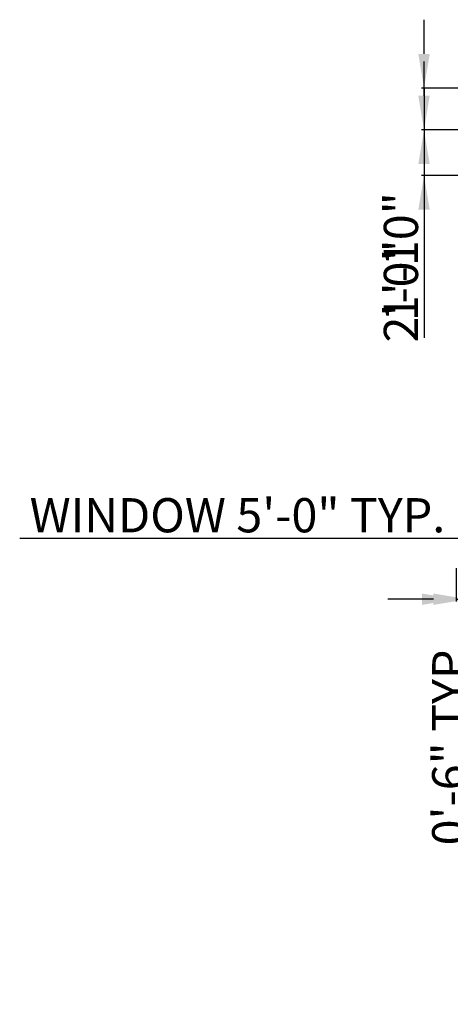
# Model space of a CAD drawing. Units: inches. Extents: x -261 to 409, y 193 to 762.
# Tile 1 of 6: x -261 to -35, y 193 to 711. Entities that reach past the tile are written whole.
import ezdxf

# ---------------------------------------------------------------- set-up
doc = ezdxf.new("R2010")
doc.units = ezdxf.units.IN
doc.layers.add('A-ANNO-DIMS', color=2, linetype='Continuous', lineweight=18)
doc.styles.get("Standard").update_dxf_attribs({"font": 'arial.ttf'})
doc.dimstyles.new('ISO-25', dxfattribs={"dimtxt": 18, "dimasz": 18, "dimexe": 1.25, "dimexo": 0.625, "dimtad": 1, "dimdec": 1, "dimlunit": 3, "dimtxsty": 'Standard', "dimcen": 2.5, "dimadec": 0, "dimazin": 0, "dimtfac": 1, "dimtdec": 1, "dimtmove": 0, "dimatfit": 3, "dimfxl": 1, "dimarcsym": 0})

# ---------------------------------------------------------------- blocks, each defined once
blk = doc.blocks.new('*D15')
at = {"layer": 'A-ANNO-DIMS', "color": 0, "lineweight": -2, "transparency": 16777216}
for p, q in [((-14.2, 438.26), (-261.22, 438.26)), ((-14.2, 429.89), (-14.2, 439.51)), ((27.8, 438.26), (3.8, 438.26)), ((45.8, 429.89), (45.8, 439.51))]:
    blk.add_line(p, q, dxfattribs=at)
at = {"layer": 'A-ANNO-DIMS', "color": 0, "transparency": 16777216}
for points in [[(3.8, 441.26), (3.8, 435.26), (-14.2, 438.26)], [(27.8, 441.26), (27.8, 435.26), (45.8, 438.26)]]:
    blk.add_solid(points, dxfattribs=at)
at = {"layer": 'Defpoints', "color": 0, "transparency": 16777216}
for p in [(-14.2, 438.26), (-14.2, 429.26), (45.8, 429.26)]:
    blk.add_point(p, dxfattribs=at)
at = {"layer": 'A-ANNO-DIMS', "color": 0, "transparency": 16777216, "insert": (-146.71, 448.2), "char_height": 18, "attachment_point": 5}
blk.add_mtext('WINDOW 5\'-0" TYP.', dxfattribs=at)
blk = doc.blocks.new('*D16')
at = {"layer": 'A-ANNO-DIMS', "color": 0, "lineweight": -2, "transparency": 16777216}
for p, q in [((-23.2, 447.26), (-23.2, 465.26)), ((-14.82, 429.26), (-24.45, 429.26)), ((-23.2, 429.26), (-23.2, 423.26)), ((-14.82, 423.26), (-24.45, 423.26)), ((-23.2, 405.26), (-23.2, 276.29))]:
    blk.add_line(p, q, dxfattribs=at)
at = {"layer": 'A-ANNO-DIMS', "color": 0, "transparency": 16777216}
for points in [[(-26.2, 447.26), (-20.2, 447.26), (-23.2, 429.26)], [(-26.2, 405.26), (-20.2, 405.26), (-23.2, 423.26)]]:
    blk.add_solid(points, dxfattribs=at)
at = {"layer": 'Defpoints', "color": 0, "transparency": 16777216}
for p in [(-14.2, 429.26), (-23.2, 423.26), (-14.2, 423.26)]:
    blk.add_point(p, dxfattribs=at)
at = {"layer": 'A-ANNO-DIMS', "color": 0, "transparency": 16777216, "insert": (-33.01, 331.78), "char_height": 18, "attachment_point": 5, "rotation": 90}
blk.add_mtext('0\'-6" TYP.', dxfattribs=at)
blk = doc.blocks.new('*D21')
at = {"layer": 'A-ANNO-DIMS', "color": 0, "lineweight": -2, "transparency": 16777216}
for p, q in [((-12.58, 537.97), (-23.96, 537.88)), ((-22.56, 519.89), (-22.27, 484.23)), ((-12, 466.31), (-23.38, 466.22)), ((-22.13, 466.23), (-19.92, 193.22))]:
    blk.add_line(p, q, dxfattribs=at)
at = {"layer": 'A-ANNO-DIMS', "color": 0, "transparency": 16777216}
for points in [[(-19.56, 519.92), (-25.56, 519.87), (-22.71, 537.89)], [(-19.27, 484.25), (-25.27, 484.2), (-22.13, 466.23)]]:
    blk.add_solid(points, dxfattribs=at)
at = {"layer": 'Defpoints', "color": 0, "transparency": 16777216}
for p in [(-11.96, 537.98), (-11.38, 466.31), (-22.13, 466.23)]:
    blk.add_point(p, dxfattribs=at)
at = {"layer": 'A-ANNO-DIMS', "color": 0, "transparency": 16777216, "insert": (-11.02, 320.8), "char_height": 18, "attachment_point": 5, "rotation": 270.4625}
blk.add_mtext('DINING SET 5\'-11 1/2"', dxfattribs=at)
blk = doc.blocks.new('*D27')
at = {"layer": 'A-ANNO-DIMS', "color": 0, "lineweight": -2, "transparency": 16777216}
for p, q in [((-31.7, 422.64), (-31.7, 405.1)), ((-14.2, 422.64), (-14.2, 405.1)), ((-49.7, 406.35), (-67.7, 406.35)), ((-31.7, 406.35), (-14.2, 406.35)), ((3.8, 406.35), (111.15, 406.35))]:
    blk.add_line(p, q, dxfattribs=at)
at = {"layer": 'A-ANNO-DIMS', "color": 0, "transparency": 16777216}
for points in [[(-49.7, 409.35), (-49.7, 403.35), (-31.7, 406.35)], [(3.8, 409.35), (3.8, 403.35), (-14.2, 406.35)]]:
    blk.add_solid(points, dxfattribs=at)
at = {"layer": 'Defpoints', "color": 0, "transparency": 16777216}
for p in [(-31.7, 423.26), (-14.2, 423.26), (-14.2, 406.35)]:
    blk.add_point(p, dxfattribs=at)
at = {"layer": 'A-ANNO-DIMS', "color": 0, "transparency": 16777216, "insert": (66.48, 416.28), "char_height": 18, "attachment_point": 5}
blk.add_mtext('1\'-5 1/2"', dxfattribs=at)
blk = doc.blocks.new('*D31')
at = {"layer": 'A-ANNO-DIMS', "color": 0, "lineweight": -2, "transparency": 16777216}
for p, q in [((-25.7, 674.64), (-25.7, 405.1)), ((-16.7, 674.64), (-16.7, 405.1)), ((-43.7, 406.35), (-61.7, 406.35)), ((-25.7, 406.35), (-16.7, 406.35)), ((1.3, 406.35), (68.4, 406.35))]:
    blk.add_line(p, q, dxfattribs=at)
at = {"layer": 'A-ANNO-DIMS', "color": 0, "transparency": 16777216}
for points in [[(-43.7, 409.35), (-43.7, 403.35), (-25.7, 406.35)], [(1.3, 409.35), (1.3, 403.35), (-16.7, 406.35)]]:
    blk.add_solid(points, dxfattribs=at)
at = {"layer": 'Defpoints', "color": 0, "transparency": 16777216}
for p in [(-25.7, 675.26), (-16.7, 675.26), (-16.7, 406.35)]:
    blk.add_point(p, dxfattribs=at)
at = {"layer": 'A-ANNO-DIMS', "color": 0, "transparency": 16777216, "insert": (43.85, 416.17), "char_height": 18, "attachment_point": 5}
blk.add_mtext('0\'-9"', dxfattribs=at)
blk = doc.blocks.new('*D35')
at = {"layer": 'A-ANNO-DIMS', "color": 0, "lineweight": -2, "transparency": 16777216}
for p, q in [((-48.61, 671.26), (-48.61, 689.26)), ((-2.32, 653.26), (-49.86, 653.26)), ((-48.61, 653.26), (-48.61, 629.26)), ((-2.32, 629.26), (-49.86, 629.26)), ((-48.61, 611.26), (-48.61, 543.86))]:
    blk.add_line(p, q, dxfattribs=at)
at = {"layer": 'A-ANNO-DIMS', "color": 0, "transparency": 16777216}
for points in [[(-51.61, 671.26), (-45.61, 671.26), (-48.61, 653.26)], [(-51.61, 611.26), (-45.61, 611.26), (-48.61, 629.26)]]:
    blk.add_solid(points, dxfattribs=at)
at = {"layer": 'Defpoints', "color": 0, "transparency": 16777216}
for p in [(-1.7, 653.26), (-48.61, 629.26), (-1.7, 629.26)]:
    blk.add_point(p, dxfattribs=at)
at = {"layer": 'A-ANNO-DIMS', "color": 0, "transparency": 16777216, "insert": (-58.42, 568.56), "char_height": 18, "attachment_point": 5, "rotation": 90}
blk.add_mtext('2\'-0"', dxfattribs=at)
blk = doc.blocks.new('*D36')
at = {"layer": 'A-ANNO-DIMS', "color": 0, "lineweight": -2, "transparency": 16777216}
for p, q in [((-25.7, 628.64), (-25.7, 405.1)), ((-1.7, 628.64), (-1.7, 405.1)), ((-43.7, 406.35), (-61.7, 406.35)), ((-25.7, 406.35), (-1.7, 406.35)), ((16.3, 406.35), (83.71, 406.35))]:
    blk.add_line(p, q, dxfattribs=at)
at = {"layer": 'A-ANNO-DIMS', "color": 0, "transparency": 16777216}
for points in [[(-43.7, 409.35), (-43.7, 403.35), (-25.7, 406.35)], [(16.3, 409.35), (16.3, 403.35), (-1.7, 406.35)]]:
    blk.add_solid(points, dxfattribs=at)
at = {"layer": 'Defpoints', "color": 0, "transparency": 16777216}
for p in [(-25.7, 629.26), (-1.7, 629.26), (-1.7, 406.35)]:
    blk.add_point(p, dxfattribs=at)
at = {"layer": 'A-ANNO-DIMS', "color": 0, "transparency": 16777216, "insert": (59.01, 416.17), "char_height": 18, "attachment_point": 5}
blk.add_mtext('2\'-0"', dxfattribs=at)
blk = doc.blocks.new('*D45')
at = {"layer": 'A-ANNO-DIMS', "color": 0, "lineweight": -2, "transparency": 16777216}
for p, q in [((-48.61, 693.26), (-48.61, 711.26)), ((-26.32, 675.26), (-49.86, 675.26)), ((-48.61, 675.26), (-48.61, 653.26)), ((-2.32, 653.26), (-49.86, 653.26)), ((-48.61, 635.26), (-48.61, 555.87))]:
    blk.add_line(p, q, dxfattribs=at)
at = {"layer": 'A-ANNO-DIMS', "color": 0, "transparency": 16777216}
for points in [[(-51.61, 693.26), (-45.61, 693.26), (-48.61, 675.26)], [(-51.61, 635.26), (-45.61, 635.26), (-48.61, 653.26)]]:
    blk.add_solid(points, dxfattribs=at)
at = {"layer": 'Defpoints', "color": 0, "transparency": 16777216}
for p in [(-25.7, 675.26), (-48.61, 653.26), (-1.7, 653.26)]:
    blk.add_point(p, dxfattribs=at)
at = {"layer": 'A-ANNO-DIMS', "color": 0, "transparency": 16777216, "insert": (-58.42, 586.57), "char_height": 18, "attachment_point": 5, "rotation": 90}
blk.add_mtext('1\'-10"', dxfattribs=at)

msp = doc.modelspace()

# ---------------------------------------------------------------- dimensions: what is measured, and where the dimension line sits
at = {"layer": 'A-ANNO-DIMS'}
for base, p1, p2, picture, middle in [((-48.61, 653.26), (-25.7, 675.26), (-1.7, 653.26), '*D45', (-58.42, 586.57)), ((-48.61, 629.26), (-1.7, 653.26), (-1.7, 629.26), '*D35', (-58.42, 568.56))]:
    dim = msp.add_linear_dim(base=base, p1=p1, p2=p2, angle=90, dimstyle='ISO-25', override={"dimdec": 1, "dimlfac": 1, "dimrnd": 0, "dimzin": 1, "dimdsep": 46, "dimlunit": 4, "dimfrac": 2}, dxfattribs=at)
    dim.commit()
    dim.dimension.update_dxf_attribs({"geometry": picture, "text_midpoint": middle})
for base, p1, p2, picture, middle in [((-16.7, 406.35), (-25.7, 675.26), (-16.7, 675.26), '*D31', (43.85, 416.17)), ((-1.7, 406.35), (-25.7, 629.26), (-1.7, 629.26), '*D36', (59.01, 416.17)), ((-14.2, 406.35), (-31.7, 423.26), (-14.2, 423.26), '*D27', (66.48, 416.28))]:
    dim = msp.add_linear_dim(base=base, p1=p1, p2=p2, dimstyle='ISO-25', override={"dimdec": 1, "dimlfac": 1, "dimrnd": 0, "dimzin": 1, "dimdsep": 46, "dimlunit": 4, "dimfrac": 2}, dxfattribs=at)
    dim.commit()
    dim.dimension.update_dxf_attribs({"geometry": picture, "text_midpoint": middle})
for base, p1, p2, angle, text, picture, middle in [((-22.13, 466.23), (-11.96, 537.98), (-11.38, 466.31), 270.4625, 'DINING SET <>', '*D21', (-11.02, 320.8)), ((-14.2, 438.26), (45.8, 429.26), (-14.2, 429.26), 180, 'WINDOW <> TYP.', '*D15', (-146.71, 448.2)), ((-23.2, 423.26), (-14.2, 429.26), (-14.2, 423.26), 270, '<> TYP.', '*D16', (-33.01, 331.78))]:
    dim = msp.add_linear_dim(base=base, p1=p1, p2=p2, angle=angle, text=text, dimstyle='ISO-25', override={"dimdec": 1, "dimlfac": 1, "dimrnd": 0, "dimzin": 1, "dimdsep": 46, "dimlunit": 4, "dimfrac": 2}, dxfattribs=at)
    dim.commit()
    dim.dimension.update_dxf_attribs({"geometry": picture, "text_midpoint": middle})

doc.saveas('drawing.dxf')
